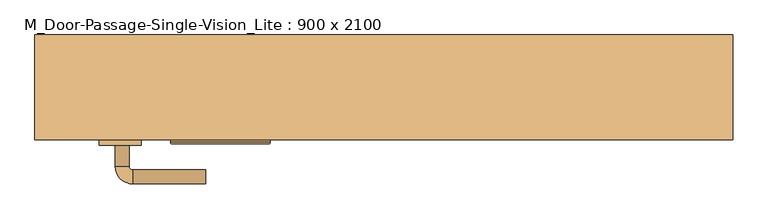
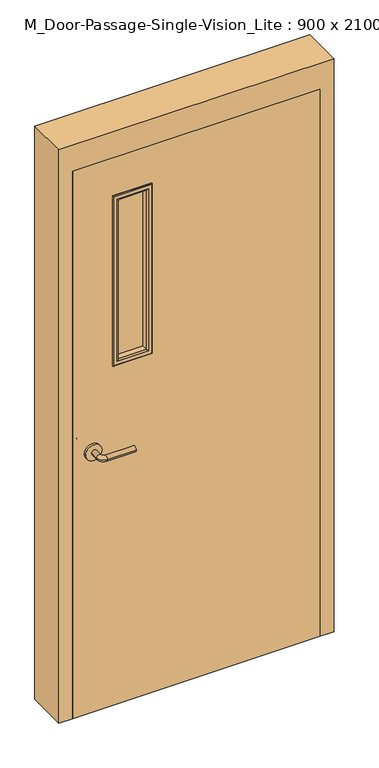
"""IFC4 building model written with IfcOpenShell, lengths in millimetres: door geometry, M_Door-Passage-Single-Vision_Lite : 900 x 2100."""

from ifc_helpers import new_model, si_unit, point, frame, frame_2d, origin, place, context, project, spatial, polyline, circle_curve, ellipse_curve, trimmed, segment, composite_curve, outline, extrude, faceted_brep, source, transform, mapped, element, save
from ifc_brep_helpers import plane_surface, cylinder_surface, revolved_surface, advanced_brep


def m_door_passage_single_vision_lite_900_x_2100_f7eb172f(model_context):
    return source(origin(), model_context, "Body", "SolidModel", [
        advanced_brep(
        [(-384.990625, -40.85, 1000.0), (-364.990625, -40.85, 1000.0), (-384.990625, -10.85, 1000.0), (-364.990625, -10.85, 1000.0), (-359.990625, -5.85, 1000.0), (-359.990625, 14.15, 1000.0), (-254.990625, 14.15, 1000.0), (-254.990625, -5.85, 1000.0)],
        [
            (0, 1, circle_curve(frame((-374.990625, -40.85, 1000.0), z_axis=(0.0, -1.0, 0.0), x_axis=(1.0, 0.0, 0.0)), 10.0)),
            (1, 0, circle_curve(frame((-374.990625, -40.85, 1000.0), z_axis=(0.0, -1.0, 0.0), x_axis=(1.0, 0.0, 0.0)), 10.0)),
            (0, 2),
            (2, 3, circle_curve(frame((-374.990625, -10.85, 1000.0), z_axis=(0.0, -1.0, 0.0), x_axis=(1.0, 0.0, 0.0)), 10.0)),
            (3, 1),
            (3, 2, circle_curve(frame((-374.990625, -10.85, 1000.0), z_axis=(0.0, -1.0, 0.0), x_axis=(1.0, 0.0, 0.0)), 10.0)),
            (4, 3, circle_curve(frame((-359.990625, -10.85, 1000.0), z_axis=(0.0, 0.0, 1.0), x_axis=(-1.0, 0.0, 0.0)), 5.0)),
            (2, 5, circle_curve(frame((-359.990625, -10.85, 1000.0), z_axis=(0.0, 0.0, -1.0), x_axis=(-1.0, 0.0, 0.0)), 25.0)),
            (5, 4, circle_curve(frame((-359.990625, 4.15, 1000.0), z_axis=(-1.0, 0.0, 0.0), x_axis=(0.0, -1.0, 0.0)), 10.0)),
            (4, 5, circle_curve(frame((-359.990625, 4.15, 1000.0), z_axis=(-1.0, 0.0, 0.0), x_axis=(0.0, -1.0, 0.0)), 10.0)),
            (6, 7, circle_curve(frame((-254.990625, 4.15, 1000.0), z_axis=(1.0, 0.0, 0.0), x_axis=(0.0, -1.0, 0.0)), 10.0)),
            (7, 6, circle_curve(frame((-254.990625, 4.15, 1000.0), z_axis=(1.0, 0.0, 0.0), x_axis=(0.0, -1.0, 0.0)), 10.0)),
            (5, 6),
            (7, 4),
        ],
        [
            plane_surface(frame((-374.990625, -40.85, 1000.0), z_axis=(0.0, -1.0, 0.0), x_axis=(0.0, 0.0, 1.0))),
            cylinder_surface(frame((-374.990625, -40.85, 1000.0), z_axis=(0.0, -1.0, 0.0), x_axis=(1.0, 0.0, 0.0)), 10.0),
            revolved_surface(trimmed(ellipse_curve(frame((-374.990625, -10.85, 1000.0), z_axis=(0.0, -1.0, 0.0), x_axis=(1.0, 0.0, 0.0)), 10.0, 10.0), [point((-384.990625, -10.85, 1000.0))], [point((-364.990625, -10.85, 1000.0))], True, "CARTESIAN"), (-359.990625, -10.85, 1000.0), (0.0, 0.0, -1.0)),
            revolved_surface(trimmed(ellipse_curve(frame((-374.990625, -10.85, 1000.0), z_axis=(0.0, -1.0, 0.0), x_axis=(1.0, 0.0, 0.0)), 10.0, 10.0), [point((-364.990625, -10.85, 1000.0))], [point((-384.990625, -10.85, 1000.0))], True, "CARTESIAN"), (-359.990625, -10.85, 1000.0), (0.0, 0.0, -1.0)),
            plane_surface(frame((-254.990625, 4.15, 1000.0), z_axis=(1.0, 0.0, 0.0), x_axis=(0.0, 0.0, 1.0))),
            cylinder_surface(frame((-359.990625, 4.15, 1000.0), z_axis=(-1.0, 0.0, 0.0), x_axis=(0.0, -1.0, 0.0)), 10.0),
        ],
        [
            (0, [[1, 2]]),
            (1, [[-1, 3, 4, 5]]),
            (1, [[-2, -5, 6, -3]]),
            (2, [[7, -4, 8, 9]]),
            (3, [[-8, -6, -7, 10]]),
            (4, [[11, 12]]),
            (5, [[-9, 13, -12, 14]]),
            (5, [[-10, -14, -11, -13]]),
        ],
    ),
        extrude(outline(composite_curve([segment(trimmed(circle_curve(frame_2d((1000.0, -377.490625)), 30.0), [point((1000.0, -407.490625))], [point((1000.0, -347.490625))], False, "CARTESIAN"), True, "CONTINUOUS"), segment(trimmed(circle_curve(frame_2d((1000.0, -377.490625)), 30.0), [point((1000.0, -347.490625))], [point((1000.0, -407.490625))], False, "CARTESIAN"), True, "CONTINUOUS")], self_intersect=False)), frame((0.0, -48.85, 0.0), z_axis=(0.0, 1.0, 0.0), x_axis=(0.0, 0.0, 1.0)), (0.0, 0.0, 1.0), 8.0),
        advanced_brep(
        [(-384.990625, -101.85, 1000.0), (-364.990625, -101.85, 1000.0), (-364.990625, -131.85, 1000.0), (-384.990625, -131.85, 1000.0), (-359.990625, -136.85, 1000.0), (-359.990625, -156.85, 1000.0), (-254.990625, -156.85, 1000.0), (-254.990625, -136.85, 1000.0)],
        [
            (0, 1, circle_curve(frame((-374.990625, -101.85, 1000.0), z_axis=(0.0, 1.0, 0.0), x_axis=(1.0, 0.0, 0.0)), 10.0)),
            (1, 0, circle_curve(frame((-374.990625, -101.85, 1000.0), z_axis=(0.0, 1.0, 0.0), x_axis=(1.0, 0.0, 0.0)), 10.0)),
            (1, 2),
            (2, 3, circle_curve(frame((-374.990625, -131.85, 1000.0), z_axis=(0.0, 1.0, 0.0), x_axis=(1.0, 0.0, 0.0)), 10.0)),
            (3, 0),
            (3, 2, circle_curve(frame((-374.990625, -131.85, 1000.0), z_axis=(0.0, 1.0, 0.0), x_axis=(1.0, 0.0, 0.0)), 10.0)),
            (4, 5, circle_curve(frame((-359.990625, -146.85, 1000.0), z_axis=(-1.0, 0.0, 0.0), x_axis=(0.0, 1.0, 0.0)), 10.0)),
            (5, 3, circle_curve(frame((-359.990625, -131.85, 1000.0), z_axis=(0.0, 0.0, -1.0), x_axis=(-1.0, 0.0, 0.0)), 25.0)),
            (2, 4, circle_curve(frame((-359.990625, -131.85, 1000.0), z_axis=(0.0, 0.0, 1.0), x_axis=(-1.0, 0.0, 0.0)), 5.0)),
            (5, 4, circle_curve(frame((-359.990625, -146.85, 1000.0), z_axis=(-1.0, 0.0, 0.0), x_axis=(0.0, 1.0, 0.0)), 10.0)),
            (6, 7, circle_curve(frame((-254.990625, -146.85, 1000.0), z_axis=(1.0, 0.0, 0.0), x_axis=(0.0, 1.0, 0.0)), 10.0)),
            (7, 6, circle_curve(frame((-254.990625, -146.85, 1000.0), z_axis=(1.0, 0.0, 0.0), x_axis=(0.0, 1.0, 0.0)), 10.0)),
            (4, 7),
            (6, 5),
        ],
        [
            plane_surface(frame((-374.990625, -101.85, 1000.0), z_axis=(0.0, 1.0, 0.0), x_axis=(0.0, 0.0, 1.0))),
            cylinder_surface(frame((-374.990625, -101.85, 1000.0), z_axis=(0.0, 1.0, 0.0), x_axis=(1.0, 0.0, 0.0)), 10.0),
            revolved_surface(trimmed(ellipse_curve(frame((-374.990625, -131.85, 1000.0), z_axis=(0.0, -1.0, 0.0), x_axis=(1.0, 0.0, 0.0)), 10.0, 10.0), [point((-384.990625, -131.85, 1000.0))], [point((-364.990625, -131.85, 1000.0))], True, "CARTESIAN"), (-359.990625, -131.85, 1000.0), (0.0, 0.0, -1.0)),
            revolved_surface(trimmed(ellipse_curve(frame((-374.990625, -131.85, 1000.0), z_axis=(0.0, -1.0, 0.0), x_axis=(1.0, 0.0, 0.0)), 10.0, 10.0), [point((-364.990625, -131.85, 1000.0))], [point((-384.990625, -131.85, 1000.0))], True, "CARTESIAN"), (-359.990625, -131.85, 1000.0), (0.0, 0.0, -1.0)),
            plane_surface(frame((-254.990625, -146.85, 1000.0), z_axis=(1.0, 0.0, 0.0), x_axis=(0.0, 0.0, 1.0))),
            cylinder_surface(frame((-359.990625, -146.85, 1000.0), z_axis=(-1.0, 0.0, 0.0), x_axis=(0.0, 1.0, 0.0)), 10.0),
        ],
        [
            (0, [[1, 2]]),
            (1, [[3, 4, 5, -2]]),
            (1, [[-5, 6, -3, -1]]),
            (2, [[7, 8, -4, 9]]),
            (3, [[10, -9, -6, -8]]),
            (4, [[11, 12]]),
            (5, [[13, -11, 14, -7]]),
            (5, [[-14, -12, -13, -10]]),
        ],
    ),
        extrude(outline(composite_curve([segment(trimmed(circle_curve(frame_2d((1000.0, -377.490625)), 30.0), [point((1000.0, -407.490625))], [point((1000.0, -347.490625))], False, "CARTESIAN"), True, "CONTINUOUS"), segment(trimmed(circle_curve(frame_2d((1000.0, -377.490625)), 30.0), [point((1000.0, -347.490625))], [point((1000.0, -407.490625))], False, "CARTESIAN"), True, "CONTINUOUS")], self_intersect=False)), frame((0.0, -101.85, 0.0), z_axis=(0.0, 1.0, 0.0), x_axis=(0.0, 0.0, 1.0)), (0.0, 0.0, 1.0), 8.0),
        extrude(outline(polyline([(2100.0, -450.0), (0.0, -450.0), (0.0, 450.0), (2100.0, 450.0), (2100.0, -450.0)]), holes=[polyline([(1947.6, -297.6), (1947.6, -170.6), (1312.6, -170.6), (1312.6, -297.6), (1947.6, -297.6)])]), frame((0.0, -93.85, 0.0), z_axis=(0.0, 1.0, 0.0), x_axis=(0.0, 0.0, 1.0)), (0.0, 0.0, 1.0), 45.0),
        faceted_brep([(450.0, -44.0875, 0.0), (434.125, -44.0875, 0.0), (434.125, 6.9375, 0.0), (450.0, 6.9375, 0.0), (450.0, 56.15, 0.0), (500.0, 56.15, 0.0), (500.0, -93.85, 0.0), (450.0, -93.85, 0.0), (450.0, -93.85, 2100.0), (450.0, -44.0875, 2100.0), (500.0, -93.85, 2200.0), (-500.0, -93.85, 2200.0), (-500.0, -93.85, 0.0), (-450.0, -93.85, 0.0), (-450.0, -93.85, 2100.0), (500.0, 56.15, 2200.0), (450.0, 56.15, 2100.0), (-450.0, 56.15, 2100.0), (-450.0, 56.15, 0.0), (-500.0, 56.15, 0.0), (-500.0, 56.15, 2200.0), (450.0, 6.9375, 2100.0), (434.125, 6.9375, 2084.125), (-434.125, 6.9375, 2084.125), (-434.125, 6.9375, 0.0), (-450.0, 6.9375, 0.0), (-450.0, 6.9375, 2100.0), (434.125, -44.0875, 2084.125), (-450.0, -44.0875, 2100.0), (-450.0, -44.0875, 0.0), (-434.125, -44.0875, 0.0), (-434.125, -44.0875, 2084.125)], [[[0, 1, 2, 3, 4, 5, 6, 7]], [[7, 8, 9, 0]], [[6, 10, 11, 12, 13, 14, 8, 7]], [[5, 15, 10, 6]], [[4, 16, 17, 18, 19, 20, 15, 5]], [[3, 21, 16, 4]], [[2, 22, 23, 24, 25, 26, 21, 3]], [[1, 27, 22, 2]], [[0, 9, 28, 29, 30, 31, 27, 1]], [[8, 14, 28, 9]], [[16, 21, 26, 17]], [[22, 27, 31, 23]], [[12, 19, 18, 25, 24, 30, 29, 13]], [[13, 29, 28, 14]], [[11, 20, 19, 12]], [[17, 26, 25, 18]], [[23, 31, 30, 24]], [[15, 20, 11, 10]]]),
        extrude(outline(polyline([(-170.6, -68.85), (-170.6, -73.85), (-297.6, -73.85), (-297.6, -68.85), (-170.6, -68.85)])), frame((0.0, 0.0, 1312.6), z_axis=(0.0, 0.0, 1.0), x_axis=(1.0, 0.0, 0.0)), (0.0, 0.0, 1.0), 635.0),
        advanced_brep(
        [(-297.6, -73.85, 1947.6), (-297.6, -73.85, 1312.6), (-297.6, -93.85, 1312.6), (-297.6, -93.85, 1947.6), (-285.6, -94.85, 1935.6), (-285.6, -94.85, 1324.6), (-285.6, -73.85, 1324.6), (-285.6, -73.85, 1935.6), (-290.6, -99.85, 1940.6), (-290.6, -99.85, 1319.6), (-305.6, -97.85, 1955.6), (-305.6, -97.85, 1304.6), (-303.6, -99.85, 1306.6), (-303.6, -99.85, 1953.6), (-305.6, -93.85, 1955.6), (-305.6, -93.85, 1304.6), (-170.6, -73.85, 1312.6), (-170.6, -93.85, 1312.6), (-182.6, -94.85, 1324.6), (-182.6, -73.85, 1324.6), (-177.6, -99.85, 1319.6), (-162.6, -97.85, 1304.6), (-164.6, -99.85, 1306.6), (-162.6, -93.85, 1304.6), (-170.6, -73.85, 1947.6), (-170.6, -93.85, 1947.6), (-182.6, -94.85, 1935.6), (-182.6, -73.85, 1935.6), (-177.6, -99.85, 1940.6), (-162.6, -97.85, 1955.6), (-164.6, -99.85, 1953.6), (-162.6, -93.85, 1955.6)],
        [
            (0, 1),
            (1, 2),
            (2, 3),
            (3, 0),
            (4, 5),
            (5, 6),
            (6, 7),
            (7, 4),
            (8, 9),
            (9, 5, ellipse_curve(frame((-290.6, -94.85, 1319.6), z_axis=(-0.7071067811865475, 0.0, 0.7071067811865475), x_axis=(0.7071067811865474, 0.0, 0.7071067811865476)), 7.0710678, 5.0)),
            (4, 8, ellipse_curve(frame((-290.6, -94.85, 1940.6), z_axis=(-0.7071067811865475, 0.0, -0.7071067811865475), x_axis=(-0.7071067811865474, 0.0, 0.7071067811865476)), 7.0710678, 5.0)),
            (10, 11),
            (11, 12, ellipse_curve(frame((-303.6, -97.85, 1306.6), z_axis=(-0.7071067811865475, 0.0, 0.7071067811865475), x_axis=(0.7071067811865474, 0.0, 0.7071067811865476)), 2.8284271, 2.0)),
            (12, 13),
            (13, 10, ellipse_curve(frame((-303.6, -97.85, 1953.6), z_axis=(-0.7071067811865475, 0.0, -0.7071067811865475), x_axis=(-0.7071067811865474, 0.0, 0.7071067811865476)), 2.8284271, 2.0)),
            (14, 15),
            (15, 11),
            (10, 14),
            (1, 16),
            (16, 17),
            (17, 2),
            (5, 18),
            (18, 19),
            (19, 6),
            (9, 20),
            (20, 18, ellipse_curve(frame((-177.6, -94.85, 1319.6), z_axis=(-0.7071067811865475, 0.0, -0.7071067811865475), x_axis=(-0.7071067811865476, 0.0, 0.7071067811865474)), 7.0710678, 5.0)),
            (11, 21),
            (21, 22, ellipse_curve(frame((-164.6, -97.85, 1306.6), z_axis=(-0.7071067811865475, 0.0, -0.7071067811865475), x_axis=(-0.7071067811865476, 0.0, 0.7071067811865474)), 2.8284271, 2.0)),
            (22, 12),
            (15, 23),
            (23, 21),
            (16, 24),
            (24, 25),
            (25, 17),
            (18, 26),
            (26, 27),
            (27, 19),
            (20, 28),
            (28, 26, ellipse_curve(frame((-177.6, -94.85, 1940.6), z_axis=(0.7071067811865475, 0.0, -0.7071067811865475), x_axis=(-0.7071067811865474, 0.0, -0.7071067811865476)), 7.0710678, 5.0)),
            (21, 29),
            (29, 30, ellipse_curve(frame((-164.6, -97.85, 1953.6), z_axis=(0.7071067811865475, 0.0, -0.7071067811865475), x_axis=(-0.7071067811865474, 0.0, -0.7071067811865476)), 2.8284271, 2.0)),
            (30, 22),
            (23, 31),
            (31, 29),
            (14, 31),
            (25, 3),
            (24, 0),
            (27, 7),
            (26, 4),
            (28, 8),
            (30, 13),
            (29, 10),
        ],
        [
            plane_surface(frame((-297.6, -93.85, 1947.6), z_axis=(-1.0, 0.0, 0.0), x_axis=(0.0, 0.0, -1.0))),
            plane_surface(frame((-285.6, -73.85, 1935.6), z_axis=(1.0, 0.0, 0.0), x_axis=(0.0, 0.0, -1.0))),
            cylinder_surface(frame((-290.6, -94.85, 1947.6), z_axis=(0.0, 0.0, 1.0), x_axis=(-1.0, 0.0, 0.0)), 5.0),
            cylinder_surface(frame((-303.6, -97.85, 1947.6), z_axis=(0.0, 0.0, 1.0), x_axis=(-1.0, 0.0, 0.0)), 2.0),
            plane_surface(frame((-305.6, -97.85, 1955.6), z_axis=(-1.0, 0.0, 0.0), x_axis=(0.0, 0.0, -1.0))),
            plane_surface(frame((-297.6, -93.85, 1312.6), z_axis=(0.0, 0.0, -1.0), x_axis=(1.0, 0.0, 0.0))),
            plane_surface(frame((-285.6, -73.85, 1324.6), z_axis=(0.0, 0.0, 1.0), x_axis=(1.0, 0.0, 0.0))),
            cylinder_surface(frame((-297.6, -94.85, 1319.6), z_axis=(-1.0, 0.0, 0.0), x_axis=(0.0, 0.0, -1.0)), 5.0),
            cylinder_surface(frame((-297.6, -97.85, 1306.6), z_axis=(-1.0, 0.0, 0.0), x_axis=(0.0, 0.0, -1.0)), 2.0),
            plane_surface(frame((-305.6, -97.85, 1304.6), z_axis=(0.0, 0.0, -1.0), x_axis=(1.0, 0.0, 0.0))),
            plane_surface(frame((-170.6, -93.85, 1312.6), z_axis=(1.0, 0.0, 0.0), x_axis=(0.0, 0.0, 1.0))),
            plane_surface(frame((-182.6, -73.85, 1324.6), z_axis=(-1.0, 0.0, 0.0), x_axis=(0.0, 0.0, 1.0))),
            cylinder_surface(frame((-177.6, -94.85, 1312.6), z_axis=(0.0, 0.0, -1.0), x_axis=(1.0, 0.0, 0.0)), 5.0),
            cylinder_surface(frame((-164.6, -97.85, 1312.6), z_axis=(0.0, 0.0, -1.0), x_axis=(1.0, 0.0, 0.0)), 2.0),
            plane_surface(frame((-162.6, -97.85, 1304.6), z_axis=(1.0, 0.0, 0.0), x_axis=(0.0, 0.0, 1.0))),
            plane_surface(frame((-162.6, -93.85, 1955.6), z_axis=(0.0, 1.0, 0.0), x_axis=(-1.0, 0.0, 0.0))),
            plane_surface(frame((-170.6, -93.85, 1947.6), z_axis=(0.0, 0.0, 1.0), x_axis=(-1.0, 0.0, 0.0))),
            plane_surface(frame((-170.6, -73.85, 1947.6), z_axis=(0.0, 1.0, 0.0), x_axis=(-1.0, 0.0, 0.0))),
            plane_surface(frame((-182.6, -73.85, 1935.6), z_axis=(0.0, 0.0, -1.0), x_axis=(-1.0, 0.0, 0.0))),
            cylinder_surface(frame((-170.6, -94.85, 1940.6), z_axis=(1.0, 0.0, 0.0), x_axis=(0.0, 0.0, 1.0)), 5.0),
            plane_surface(frame((-177.6, -99.85, 1940.6), z_axis=(0.0, -1.0, 0.0), x_axis=(-1.0, 0.0, 0.0))),
            cylinder_surface(frame((-170.6, -97.85, 1953.6), z_axis=(1.0, 0.0, 0.0), x_axis=(0.0, 0.0, 1.0)), 2.0),
            plane_surface(frame((-162.6, -97.85, 1955.6), z_axis=(0.0, 0.0, 1.0), x_axis=(-1.0, 0.0, 0.0))),
        ],
        [
            (0, [[1, 2, 3, 4]]),
            (1, [[5, 6, 7, 8]]),
            (2, [[9, 10, -5, 11]]),
            (3, [[12, 13, 14, 15]]),
            (4, [[16, 17, -12, 18]]),
            (5, [[19, 20, 21, -2]]),
            (6, [[22, 23, 24, -6]]),
            (7, [[25, 26, -22, -10]]),
            (8, [[27, 28, 29, -13]]),
            (9, [[30, 31, -27, -17]]),
            (10, [[32, 33, 34, -20]]),
            (11, [[35, 36, 37, -23]]),
            (12, [[38, 39, -35, -26]]),
            (13, [[40, 41, 42, -28]]),
            (14, [[43, 44, -40, -31]]),
            (15, [[-16, 45, -43, -30], [-3, -21, -34, 46]]),
            (16, [[47, -4, -46, -33]]),
            (17, [[-1, -47, -32, -19], [-7, -24, -37, 48]]),
            (18, [[49, -8, -48, -36]]),
            (19, [[50, -11, -49, -39]]),
            (20, [[-14, -29, -42, 51], [-9, -50, -38, -25]]),
            (21, [[52, -15, -51, -41]]),
            (22, [[-45, -18, -52, -44]]),
        ],
    ),
        advanced_brep(
        [(-297.6, -68.85, 1312.6), (-297.6, -68.85, 1947.6), (-297.6, -48.85, 1947.6), (-297.6, -48.85, 1312.6), (-285.6, -47.85, 1324.6), (-285.6, -47.85, 1935.6), (-285.6, -68.85, 1935.6), (-285.6, -68.85, 1324.6), (-290.6, -42.85, 1319.6), (-290.6, -42.85, 1940.6), (-305.6, -44.85, 1304.6), (-305.6, -44.85, 1955.6), (-303.6, -42.85, 1953.6), (-303.6, -42.85, 1306.6), (-305.6, -48.85, 1304.6), (-305.6, -48.85, 1955.6), (-170.6, -68.85, 1947.6), (-170.6, -48.85, 1947.6), (-182.6, -47.85, 1935.6), (-182.6, -68.85, 1935.6), (-177.6, -42.85, 1940.6), (-162.6, -44.85, 1955.6), (-164.6, -42.85, 1953.6), (-162.6, -48.85, 1955.6), (-170.6, -68.85, 1312.6), (-170.6, -48.85, 1312.6), (-182.6, -47.85, 1324.6), (-182.6, -68.85, 1324.6), (-177.6, -42.85, 1319.6), (-162.6, -44.85, 1304.6), (-164.6, -42.85, 1306.6), (-162.6, -48.85, 1304.6)],
        [
            (0, 1),
            (1, 2),
            (2, 3),
            (3, 0),
            (4, 5),
            (5, 6),
            (6, 7),
            (7, 4),
            (8, 9),
            (9, 5, ellipse_curve(frame((-290.6, -47.85, 1940.6), z_axis=(-0.7071067811865475, 0.0, -0.7071067811865475), x_axis=(0.7071067811865474, 0.0, -0.7071067811865476)), 7.0710678, 5.0)),
            (4, 8, ellipse_curve(frame((-290.6, -47.85, 1319.6), z_axis=(-0.7071067811865475, 0.0, 0.7071067811865475), x_axis=(-0.7071067811865474, 0.0, -0.7071067811865476)), 7.0710678, 5.0)),
            (10, 11),
            (11, 12, ellipse_curve(frame((-303.6, -44.85, 1953.6), z_axis=(-0.7071067811865475, 0.0, -0.7071067811865475), x_axis=(0.7071067811865474, 0.0, -0.7071067811865476)), 2.8284271, 2.0)),
            (12, 13),
            (13, 10, ellipse_curve(frame((-303.6, -44.85, 1306.6), z_axis=(-0.7071067811865475, 0.0, 0.7071067811865475), x_axis=(-0.7071067811865474, 0.0, -0.7071067811865476)), 2.8284271, 2.0)),
            (14, 15),
            (15, 11),
            (10, 14),
            (1, 16),
            (16, 17),
            (17, 2),
            (5, 18),
            (18, 19),
            (19, 6),
            (9, 20),
            (20, 18, ellipse_curve(frame((-177.6, -47.85, 1940.6), z_axis=(-0.7071067811865475, 0.0, 0.7071067811865475), x_axis=(-0.7071067811865476, 0.0, -0.7071067811865474)), 7.0710678, 5.0)),
            (11, 21),
            (21, 22, ellipse_curve(frame((-164.6, -44.85, 1953.6), z_axis=(-0.7071067811865475, 0.0, 0.7071067811865475), x_axis=(-0.7071067811865476, 0.0, -0.7071067811865474)), 2.8284271, 2.0)),
            (22, 12),
            (15, 23),
            (23, 21),
            (16, 24),
            (24, 25),
            (25, 17),
            (18, 26),
            (26, 27),
            (27, 19),
            (20, 28),
            (28, 26, ellipse_curve(frame((-177.6, -47.85, 1319.6), z_axis=(0.7071067811865475, 0.0, 0.7071067811865475), x_axis=(-0.7071067811865474, 0.0, 0.7071067811865476)), 7.0710678, 5.0)),
            (21, 29),
            (29, 30, ellipse_curve(frame((-164.6, -44.85, 1306.6), z_axis=(0.7071067811865475, 0.0, 0.7071067811865475), x_axis=(-0.7071067811865474, 0.0, 0.7071067811865476)), 2.8284271, 2.0)),
            (30, 22),
            (23, 31),
            (31, 29),
            (14, 31),
            (25, 3),
            (24, 0),
            (27, 7),
            (26, 4),
            (28, 8),
            (30, 13),
            (29, 10),
        ],
        [
            plane_surface(frame((-297.6, -48.85, 1312.6), z_axis=(-1.0, 0.0, 0.0), x_axis=(0.0, 0.0, 1.0))),
            plane_surface(frame((-285.6, -68.85, 1324.6), z_axis=(1.0, 0.0, 0.0), x_axis=(0.0, 0.0, 1.0))),
            cylinder_surface(frame((-290.6, -47.85, 1312.6), z_axis=(0.0, 0.0, -1.0), x_axis=(-1.0, 0.0, 0.0)), 5.0),
            cylinder_surface(frame((-303.6, -44.85, 1312.6), z_axis=(0.0, 0.0, -1.0), x_axis=(-1.0, 0.0, 0.0)), 2.0),
            plane_surface(frame((-305.6, -44.85, 1304.6), z_axis=(-1.0, 0.0, 0.0), x_axis=(0.0, 0.0, 1.0))),
            plane_surface(frame((-297.6, -48.85, 1947.6), z_axis=(0.0, 0.0, 1.0), x_axis=(1.0, 0.0, 0.0))),
            plane_surface(frame((-285.6, -68.85, 1935.6), z_axis=(0.0, 0.0, -1.0), x_axis=(1.0, 0.0, 0.0))),
            cylinder_surface(frame((-297.6, -47.85, 1940.6), z_axis=(-1.0, 0.0, 0.0), x_axis=(0.0, 0.0, 1.0)), 5.0),
            cylinder_surface(frame((-297.6, -44.85, 1953.6), z_axis=(-1.0, 0.0, 0.0), x_axis=(0.0, 0.0, 1.0)), 2.0),
            plane_surface(frame((-305.6, -44.85, 1955.6), z_axis=(0.0, 0.0, 1.0), x_axis=(1.0, 0.0, 0.0))),
            plane_surface(frame((-170.6, -48.85, 1947.6), z_axis=(1.0, 0.0, 0.0), x_axis=(0.0, 0.0, -1.0))),
            plane_surface(frame((-182.6, -68.85, 1935.6), z_axis=(-1.0, 0.0, 0.0), x_axis=(0.0, 0.0, -1.0))),
            cylinder_surface(frame((-177.6, -47.85, 1947.6), z_axis=(0.0, 0.0, 1.0), x_axis=(1.0, 0.0, 0.0)), 5.0),
            cylinder_surface(frame((-164.6, -44.85, 1947.6), z_axis=(0.0, 0.0, 1.0), x_axis=(1.0, 0.0, 0.0)), 2.0),
            plane_surface(frame((-162.6, -44.85, 1955.6), z_axis=(1.0, 0.0, 0.0), x_axis=(0.0, 0.0, -1.0))),
            plane_surface(frame((-162.6, -48.85, 1304.6), z_axis=(0.0, -1.0, 0.0), x_axis=(-1.0, 0.0, 0.0))),
            plane_surface(frame((-170.6, -48.85, 1312.6), z_axis=(0.0, 0.0, -1.0), x_axis=(-1.0, 0.0, 0.0))),
            plane_surface(frame((-170.6, -68.85, 1312.6), z_axis=(0.0, -1.0, 0.0), x_axis=(-1.0, 0.0, 0.0))),
            plane_surface(frame((-182.6, -68.85, 1324.6), z_axis=(0.0, 0.0, 1.0), x_axis=(-1.0, 0.0, 0.0))),
            cylinder_surface(frame((-170.6, -47.85, 1319.6), z_axis=(1.0, 0.0, 0.0), x_axis=(0.0, 0.0, -1.0)), 5.0),
            plane_surface(frame((-177.6, -42.85, 1319.6), z_axis=(0.0, 1.0, 0.0), x_axis=(-1.0, 0.0, 0.0))),
            cylinder_surface(frame((-170.6, -44.85, 1306.6), z_axis=(1.0, 0.0, 0.0), x_axis=(0.0, 0.0, -1.0)), 2.0),
            plane_surface(frame((-162.6, -44.85, 1304.6), z_axis=(0.0, 0.0, -1.0), x_axis=(-1.0, 0.0, 0.0))),
        ],
        [
            (0, [[1, 2, 3, 4]]),
            (1, [[5, 6, 7, 8]]),
            (2, [[9, 10, -5, 11]]),
            (3, [[12, 13, 14, 15]]),
            (4, [[16, 17, -12, 18]]),
            (5, [[19, 20, 21, -2]]),
            (6, [[22, 23, 24, -6]]),
            (7, [[25, 26, -22, -10]]),
            (8, [[27, 28, 29, -13]]),
            (9, [[30, 31, -27, -17]]),
            (10, [[32, 33, 34, -20]]),
            (11, [[35, 36, 37, -23]]),
            (12, [[38, 39, -35, -26]]),
            (13, [[40, 41, 42, -28]]),
            (14, [[43, 44, -40, -31]]),
            (15, [[-16, 45, -43, -30], [-3, -21, -34, 46]]),
            (16, [[47, -4, -46, -33]]),
            (17, [[-1, -47, -32, -19], [-7, -24, -37, 48]]),
            (18, [[49, -8, -48, -36]]),
            (19, [[50, -11, -49, -39]]),
            (20, [[-14, -29, -42, 51], [-9, -50, -38, -25]]),
            (21, [[52, -15, -51, -41]]),
            (22, [[-45, -18, -52, -44]]),
        ],
    ),
    ])


if __name__ == "__main__":
    model = new_model("IFC4")
    model_context = context("Model", 3, world=origin())
    ifc_project = project(units=[si_unit("LENGTHUNIT", "METRE", prefix="MILLI")], contexts=[model_context])
    site = spatial("IfcSite", under=ifc_project)
    building = spatial("IfcBuilding", under=site)
    placement = place(None, origin())
    m_door_passage_single_vision_lite_900_x_2100_shape = m_door_passage_single_vision_lite_900_x_2100_f7eb172f(model_context)
    element("IfcDoor", 1, ObjectType="M_Door-Passage-Single-Vision_Lite : 900 x 2100", at=placement, inside=building, context=model_context, shape_type="MappedRepresentation", body=[
        mapped(m_door_passage_single_vision_lite_900_x_2100_shape, transform((0.0, 0.0, 0.0), x_axis=(1.0, 0.0, 0.0), y_axis=(0.0, 1.0, 0.0), z_axis=(0.0, 0.0, 1.0))),
    ])
    save(model, "model.ifc")

# Revit data of these elements
# Type "M_Door-Passage-Single-Vision_Lite : 900 x 2100"
#   Type Mark = "46"
#   Assembly Code = "B2030100"
#   Analytic Construction = "Wooden"
#   Thickness = 45 mm
#   Thermal Resistance (R) = 0.455703 (m²·K)/W
#   Swing Angle [instance default] = 90.00°
#   Strike Height = 1000 mm
#   Rough Width [instance default] = 1000 mm
#   Rough Height [instance default] = 2200 mm
#   MFOpeningHeight [instance default] = 100 mm
#   MFOpeningWidth [instance default] = 100 mm
#   Inset Calculate [instance default] = 105 mm
#   Masonry Inset [instance default] = 25 mm
#   Height = 2100 mm
#   Width = 900 mm
#   Heat Transfer Coefficient (U) = 2.19465 W/(m²·K)
#   Masonry Frame Depth = 150 mm
#   Masonry Frame [instance default] = yes
#   Function = 1
#   Dry Wall Frame [instance default] = no
#   Panel Material = Wood - Birch
#   Glazing = Glass
#   Glass Stop Material = Metal - Paint Finish - Grey
#   Frame Material = Metal - Paint Finish - Grey
#   Door Handle Material = Aluminum
#   Visual Light Transmittance = 0
#   Solar Heat Gain Coefficient = 0
#   Wall Closure = (empty or 0)
# Element 1 (IfcDoor, "M_Door-Passage-Single-Vision_Lite : 900 x 2100")
#   Materials on its faces: "Metal - Paint Finish - Grey", "Aluminum", "Wood - Birch", "Glass"
# Materials
#   "Wood - Birch": class "Wood", colour RGB 173 132 96, transparency 0, Cost = 0
#   "Glass": class "Glass", colour RGB 245 245 243, transparency 1, Description = "Soda Lime Glass", Cost = 0
#   "Metal - Paint Finish - Grey": class "Paint", colour RGB 178 178 178, transparency 0, Cost = 0
#   "Aluminum": class "Metal", colour RGB 244 245 246, transparency 0, Description = "Aluminum 6061", Cost = 0
